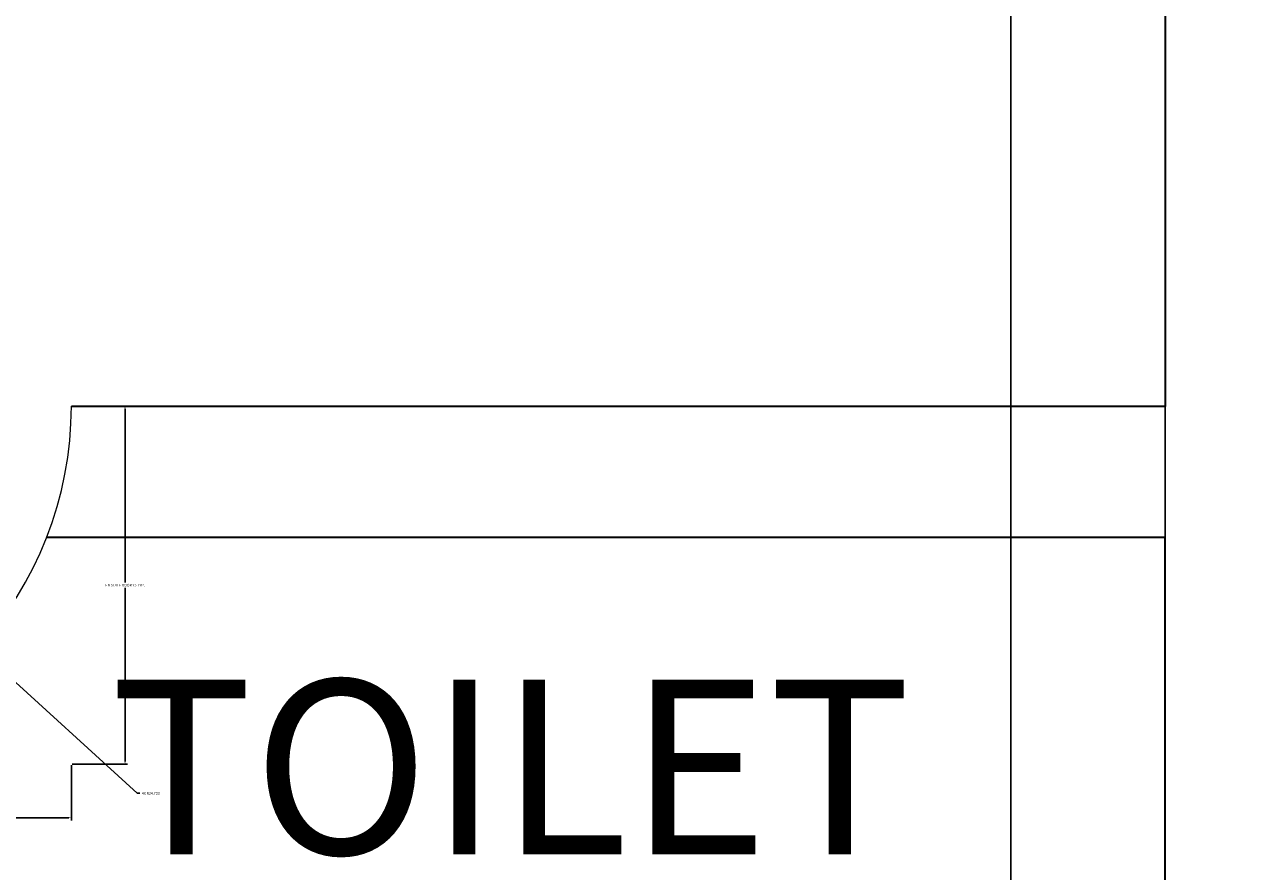
# Model space of a CAD drawing. Units: feet. Extents: x 5816 to 6644, y 25475 to 26788.
# Tile 21 of 23: x 6147 to 6232, y 26536 to 26594. Entities that reach past the tile are written whole.
import ezdxf

# ---------------------------------------------------------------- set-up
doc = ezdxf.new("R2010")
doc.units = ezdxf.units.FT
for name, color, linetype, lineweight in [('A-ANNO-DIMS', 2, 'Continuous', 13), ('A-AREA-IDEN', 7, 'Continuous', 18), ('A-DOOR', 3, 'Continuous', 18), ('A-WALL', 7, 'Continuous', 35)]:
    doc.layers.add(name, color=color, linetype=linetype, lineweight=lineweight)
doc.styles.get("Standard").update_dxf_attribs({"font": 'arial.ttf'})
doc.dimstyles.get("Standard").update_dxf_attribs({"dimtxt": 0.18, "dimasz": 0.18, "dimexe": 0.18, "dimexo": 0.0625, "dimgap": 0.09, "dimtad": 0, "dimtih": 1, "dimtoh": 1, "dimdec": 4, "dimzin": 0, "dimdsep": 46, "dimtxsty": 'Standard', "dimcen": 0.09, "dimadec": 0, "dimazin": 0, "dimtfac": 1, "dimtdec": 4, "dimtofl": 0, "dimtmove": 0, "dimatfit": 3, "dimfxl": 1, "dimtolj": 1, "dimtzin": 0, "dimarcsym": 0})

# ---------------------------------------------------------------- blocks, each defined once
blk = doc.blocks.new('DOOR-BATH-ENSUITE')
blk.add_line((0, -24.59), (0, 0))
blk.add_arc((-2.33, 0.023), 24.723, 275.40734, 0)
blk = doc.blocks.new('*D33')
at = {"layer": 'A-ANNO-DIMS', "color": 0, "lineweight": -2, "transparency": 16777216}
for p, q in [((6150.144, 26567.608), (6153.953, 26567.608)), ((6153.773, 26567.428), (6153.773, 26555.485)), ((6153.773, 26543.175), (6153.773, 26555.118)), ((6150.144, 26542.995), (6153.953, 26542.995))]:
    blk.add_line(p, q, dxfattribs=at)
at = {"layer": 'A-ANNO-DIMS', "color": 0, "transparency": 16777216}
for points in [[(6153.743, 26567.428), (6153.803, 26567.428), (6153.773, 26567.608)], [(6153.743, 26543.175), (6153.803, 26543.175), (6153.773, 26542.995)]]:
    blk.add_solid(points, dxfattribs=at)
at = {"layer": 'Defpoints', "color": 0, "transparency": 16777216}
for p in [(6150.081, 26567.608), (6153.773, 26567.608), (6150.081, 26542.995)]:
    blk.add_point(p, dxfattribs=at)
at = {"layer": 'A-ANNO-DIMS', "color": 0, "transparency": 16777216, "insert": (6153.773, 26555.301), "char_height": 0.18, "attachment_point": 5}
blk.add_mtext('\\A1;EN SUITE DOOR 25 TYP.', dxfattribs=at)
blk = doc.blocks.new('*D34')
at = {"layer": 'A-ANNO-DIMS', "color": 0, "lineweight": -2, "transparency": 16777216}
for p, q in [((6127.688, 26542.932), (6127.688, 26539.123)), ((6150.081, 26542.932), (6150.081, 26539.123)), ((6127.868, 26539.303), (6138.355, 26539.303)), ((6149.901, 26539.303), (6139.414, 26539.303))]:
    blk.add_line(p, q, dxfattribs=at)
at = {"layer": 'A-ANNO-DIMS', "color": 0, "transparency": 16777216}
for points in [[(6127.868, 26539.333), (6127.868, 26539.273), (6127.688, 26539.303)], [(6149.901, 26539.333), (6149.901, 26539.273), (6150.081, 26539.303)]]:
    blk.add_solid(points, dxfattribs=at)
at = {"layer": 'Defpoints', "color": 0, "transparency": 16777216}
for p in [(6127.688, 26542.995), (6150.081, 26542.995), (6150.081, 26539.303)]:
    blk.add_point(p, dxfattribs=at)
at = {"layer": 'A-ANNO-DIMS', "color": 0, "transparency": 16777216, "insert": (6138.884, 26539.303), "char_height": 0.18, "attachment_point": 5}
blk.add_mtext('\\A1;22 TYP.', dxfattribs=at)
blk = doc.blocks.new('*D60')
at = {"layer": 'A-ANNO-DIMS', "color": 0, "lineweight": -2, "transparency": 16777216}
for p, q in [((6106.978, 26094.399), (6106.978, 26787.915)), ((6107.158, 26787.735), (6224.932, 26787.735)), ((6343.496, 26787.735), (6225.722, 26787.735)), ((6343.676, 26094.399), (6343.676, 26787.915))]:
    blk.add_line(p, q, dxfattribs=at)
at = {"layer": 'A-ANNO-DIMS', "color": 0, "transparency": 16777216}
for points in [[(6107.158, 26787.765), (6107.158, 26787.705), (6106.978, 26787.735)], [(6343.496, 26787.765), (6343.496, 26787.705), (6343.676, 26787.735)]]:
    blk.add_solid(points, dxfattribs=at)
at = {"layer": 'Defpoints', "color": 0, "transparency": 16777216}
for p in [(6343.676, 26787.735), (6106.978, 26094.337), (6343.676, 26094.337)]:
    blk.add_point(p, dxfattribs=at)
at = {"layer": 'A-ANNO-DIMS', "color": 0, "transparency": 16777216, "insert": (6225.327, 26787.735), "char_height": 0.18, "attachment_point": 5}
blk.add_mtext('\\A1;236.7', dxfattribs=at)
blk = doc.blocks.new('*D72')
at = {"layer": 'A-ANNO-DIMS', "color": 0, "lineweight": -2, "transparency": 16777216}
for p, q in [((6214.691, 26168.647), (6214.691, 26787.915)), ((6214.871, 26787.735), (6219.563, 26787.735)), ((6225.132, 26787.735), (6220.439, 26787.735)), ((6225.312, 26177.647), (6225.312, 26787.915))]:
    blk.add_line(p, q, dxfattribs=at)
at = {"layer": 'A-ANNO-DIMS', "color": 0, "transparency": 16777216}
for points in [[(6214.871, 26787.765), (6214.871, 26787.705), (6214.691, 26787.735)], [(6225.132, 26787.765), (6225.132, 26787.705), (6225.312, 26787.735)]]:
    blk.add_solid(points, dxfattribs=at)
at = {"layer": 'Defpoints', "color": 0, "transparency": 16777216}
for p in [(6225.312, 26787.735), (6225.312, 26177.585), (6214.691, 26168.585)]:
    blk.add_point(p, dxfattribs=at)
at = {"layer": 'A-ANNO-DIMS', "color": 0, "transparency": 16777216, "insert": (6220.001, 26787.735), "char_height": 0.18, "attachment_point": 5}
blk.add_mtext('\\A1;10.621', dxfattribs=at)
blk = doc.blocks.new('*D80')
at = {"layer": 'A-ANNO-DIMS', "color": 0, "lineweight": -2, "transparency": 16777216}
for p, q in [((6125.268, 26567.608), (6125.448, 26567.608)), ((6125.358, 26567.518), (6125.358, 26567.698)), ((6154.617, 26540.987), (6143.778, 26550.849)), ((6154.797, 26540.987), (6154.617, 26540.987))]:
    blk.add_line(p, q, dxfattribs=at)
at = {"layer": 'A-ANNO-DIMS', "color": 0, "transparency": 16777216}
blk.add_solid([(6143.798, 26550.871), (6143.758, 26550.827), (6143.645, 26550.97)], dxfattribs=at)
at = {"layer": 'Defpoints', "color": 0, "transparency": 16777216}
for p in [(6125.358, 26567.608), (6143.645, 26550.97)]:
    blk.add_point(p, dxfattribs=at)
at = {"layer": 'A-ANNO-DIMS', "color": 0, "transparency": 16777216, "insert": (6155.544, 26540.987), "char_height": 0.18, "attachment_point": 5}
blk.add_mtext('\\A1;4X R24.723', dxfattribs=at)

msp = doc.modelspace()

# ---------------------------------------------------------------- linework, layer by layer
at = {"layer": 'A-WALL'}
for p, q in [((6225.3119, 26717.5846), (6225.3119, 26567.5846)), ((6225.3119, 26567.5846), (6150.0811, 26567.5846)), ((6225.3119, 26558.5846), (6148.3757, 26558.5846)), ((6225.3119, 26558.5846), (6148.3757, 26558.5846)), ((6225.3119, 26507.5846), (6225.3119, 26558.5846))]:
    msp.add_line(p, q, dxfattribs=at)

# ---------------------------------------------------------------- block references
at = {"layer": 'A-DOOR'}
msp.add_blockref('DOOR-BATH-ENSUITE', (6127.6877, 26567.5846), dxfattribs=at)

# ---------------------------------------------------------------- texts
at = {"layer": 'A-AREA-IDEN'}
msp.add_text('TOILET', height=12, dxfattribs=at).set_placement((6152.7543, 26536.7929))

# ---------------------------------------------------------------- dimensions: what is measured, and where the dimension line sits
at = {"layer": 'A-ANNO-DIMS'}
for base, p1, p2, override, picture, middle in [((6343.6763, 26787.7346), (6106.9781, 26094.3368), (6343.6763, 26094.3368), {"dimdec": 1, "dimlfac": 1, "dimrnd": 0, "dimzin": 0, "dimdsep": 46, "dimlunit": 2}, '*D60', (6225.3272, 26787.7346)), ((6225.3119, 26787.7346), (6214.6905, 26168.5846), (6225.3119, 26177.5846), {"dimdec": 3, "dimlfac": 1, "dimrnd": 0, "dimzin": 0, "dimdsep": 46, "dimlunit": 2}, '*D72', (6220.0012, 26787.7346))]:
    dim = msp.add_linear_dim(base=base, p1=p1, p2=p2, dimstyle='Standard', override=override, dxfattribs=at)
    dim.commit()
    dim.dimension.update_dxf_attribs({"geometry": picture, "text_midpoint": middle})
dim = msp.add_radius_dim(center=(6125.3579, 26567.608), mpoint=(6143.645, 26550.97), text='4X <>', dimstyle='Standard', override={"dimdec": 3, "dimlfac": 1, "dimrnd": 0, "dimzin": 0, "dimdsep": 46, "dimlunit": 2}, dxfattribs=at)
dim.commit()
dim.dimension.update_dxf_attribs({"geometry": '*D80', "text_midpoint": (6155.544, 26540.9872), "dimtype": 164})
dim = msp.add_linear_dim(base=(6153.7731, 26567.608), p1=(6150.0811, 26542.9948), p2=(6150.0811, 26567.608), angle=90, text='EN SUITE DOOR <> TYP.', dimstyle='Standard', override={"dimdec": 0, "dimlfac": 1, "dimrnd": 0, "dimzin": 0, "dimdsep": 46, "dimlunit": 2}, dxfattribs=at)
dim.commit()
dim.dimension.update_dxf_attribs({"geometry": '*D33', "text_midpoint": (6153.7731, 26555.3014)})
dim = msp.add_linear_dim(base=(6150.0811, 26539.3028), p1=(6127.6877, 26542.9948), p2=(6150.0811, 26542.9948), text='<> TYP.', dimstyle='Standard', override={"dimdec": 0, "dimlfac": 1, "dimrnd": 0, "dimzin": 0, "dimdsep": 46, "dimlunit": 2}, dxfattribs=at)
dim.commit()
dim.dimension.update_dxf_attribs({"geometry": '*D34', "text_midpoint": (6138.8844, 26539.3028)})

doc.saveas('drawing.dxf')
